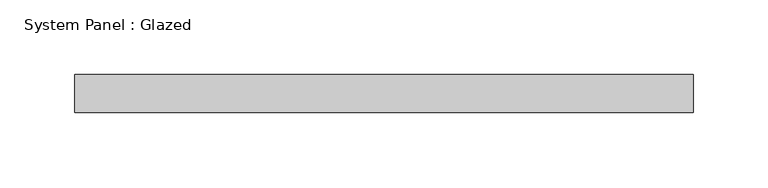
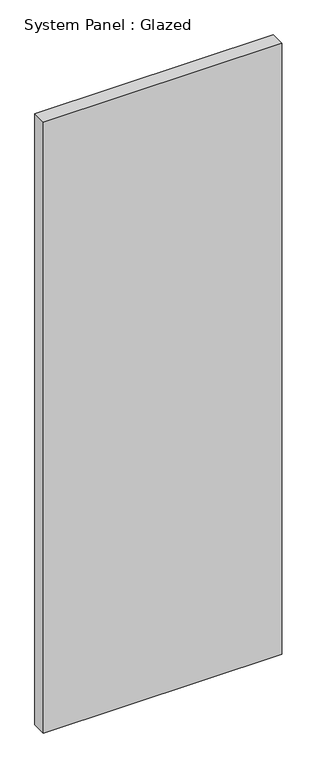
"""IFC4 building model written with IfcOpenShell, lengths in millimetres: plate geometry, System Panel : Glazed."""

from ifc_helpers import new_model, si_unit, origin, origin_with_axes, place, context, project, spatial, polyline, outline, extrude, source, transform, mapped, element, save


def system_panel_glazed_d052c37f(model_context):
    return source(origin(), model_context, "Body", "SweptSolid", [
        extrude(outline(polyline([(206.375, 19.05), (-206.375, 19.05), (-206.375, 44.45), (206.375, 44.45), (206.375, 19.05)])), origin_with_axes(), (0.0, 0.0, 1.0), 1117.6),
    ])


if __name__ == "__main__":
    model = new_model("IFC4")
    model_context = context("Model", 3, world=origin())
    ifc_project = project(units=[si_unit("LENGTHUNIT", "METRE", prefix="MILLI")], contexts=[model_context])
    site = spatial("IfcSite", under=ifc_project)
    building = spatial("IfcBuilding", under=site)
    placement = place(None, origin())
    system_panel_glazed_shape = system_panel_glazed_d052c37f(model_context)
    element("IfcPlate", 1, ObjectType="System Panel : Glazed", at=placement, inside=building, context=model_context, shape_type="MappedRepresentation", body=[
        mapped(system_panel_glazed_shape, transform((0.0, 0.0, 0.0), x_axis=(1.0, 0.0, 0.0), y_axis=(0.0, 1.0, 0.0), z_axis=(0.0, 0.0, 1.0))),
    ])
    save(model, "model.ifc")

# Revit data of these elements
# Type "System Panel : Glazed"
#   Construction Type Id = "GSP4R"
#   Analytic Construction = "1/8 in Pilkington single glazing"
#   Visual Light Transmittance = 0.9
#   Solar Heat Gain Coefficient = 0.86
#   Heat Transfer Coefficient (U) = 1.18115 BTU/(h·ft²·°F)
#   Define Thermal Properties by = 1
# Element 1 (IfcPlate, "System Panel : Glazed")
#   Materials on its faces: "Glass"
# Materials
#   "Glass": class "Glass", colour RGB 0 128 192, transparency 0.75, Description = "Soda Lime Glass", Cost = 0
